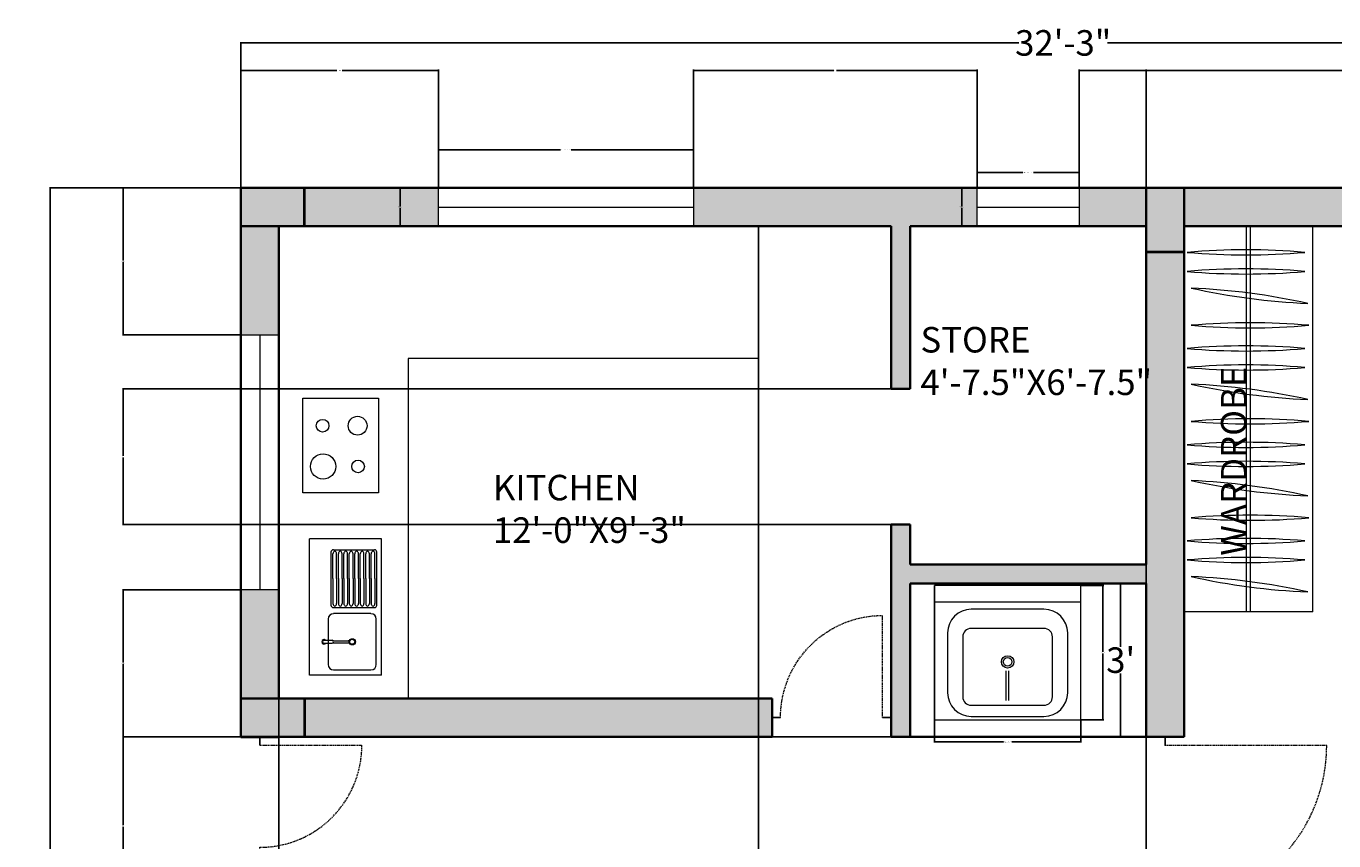
# Model space of a CAD drawing. Units: inches. Extents: x -10 to 455, y -513 to 57.
# Tile 3 of 4: x -10 to 297, y -134 to 57. Entities that reach past the tile are written whole.
import ezdxf

# ---------------------------------------------------------------- set-up
doc = ezdxf.new("R2010")
doc.units = ezdxf.units.IN
doc.header["$MEASUREMENT"] = 0
doc.linetypes.add('DASHED2', pattern=[0.375, 0.25, -0.125])
for name, color, linetype, lineweight in [('A-ANNO-DIMS', 2, 'Continuous', 18), ('A-ANNO-TEXT', 7, 'Continuous', 18), ('A-AREA-IDEN', 7, 'Continuous', 18), ('A-COLS', 7, 'Continuous', 40), ('A-COLS-PATT', 1, 'Continuous', 13), ('A-DOOR', 40, 'DASHED2', 18), ('A-DOOR-FRAM', 7, 'Continuous', 25), ('A-EQPM', 9, 'Continuous', 18), ('A-FLOR-CASE', 8, 'Continuous', 18), ('A-FLOR-FIXT', 9, 'Continuous', 18), ('A-GLAZ', 222, 'Continuous', 18), ('A-WALL', 7, 'Continuous', 35), ('A-WALL-PATT', 152, 'Continuous', 13)]:
    doc.layers.add(name, color=color, linetype=linetype, lineweight=lineweight)
doc.styles.get("Standard").update_dxf_attribs({"font": 'arial.ttf'})
doc.dimstyles.get("Standard").update_dxf_attribs({"dimtxt": 0.18, "dimasz": 0.18, "dimexe": 0.18, "dimexo": 0.0625, "dimgap": 0.09, "dimtad": 0, "dimtih": 1, "dimtoh": 1, "dimdec": 0, "dimzin": 0, "dimdsep": 46, "dimlunit": 3, "dimtxsty": 'Standard', "dimcen": 0.09, "dimadec": 0, "dimazin": 0, "dimtfac": 1, "dimtdec": 0, "dimtofl": 0, "dimtmove": 0, "dimatfit": 3, "dimfxl": 1, "dimtolj": 1, "dimtzin": 0, "dimarcsym": 0})

# ---------------------------------------------------------------- blocks, each defined once
blk = doc.blocks.new('*D1')
at = {"layer": 'A-ANNO-DIMS', "color": 0, "lineweight": -2, "transparency": 16777216}
for p, q in [((40.25, 19.21), (40.25, 53.43)), ((40.43, 53.25), (223.35, 53.25)), ((427.07, 53.25), (244.14, 53.25)), ((427.25, 19.21), (427.25, 53.43))]:
    blk.add_line(p, q, dxfattribs=at)
at = {"layer": 'A-ANNO-DIMS', "color": 0, "transparency": 16777216}
for points in [[(40.43, 53.28), (40.43, 53.22), (40.25, 53.25)], [(427.07, 53.28), (427.07, 53.22), (427.25, 53.25)]]:
    blk.add_solid(points, dxfattribs=at)
at = {"layer": 'Defpoints', "color": 0, "transparency": 16777216}
for p in [(427.25, 53.25), (40.25, 19.15), (427.25, 19.15)]:
    blk.add_point(p, dxfattribs=at)
at = {"layer": 'A-ANNO-DIMS', "color": 0, "transparency": 16777216, "insert": (233.75, 53.25), "char_height": 6, "attachment_point": 5}
blk.add_mtext('\\A1;32\'-3"', dxfattribs=at)
blk = doc.blocks.new('*D2')
at = {"layer": 'A-ANNO-DIMS', "color": 0, "lineweight": -2, "transparency": 16777216}
for p, q in [((40.18, 19.15), (-4.74, 19.15)), ((-4.56, 18.97), (-4.56, -229.75)), ((-4.56, -484.67), (-4.56, -235.95)), ((40.18, -484.85), (-4.74, -484.85))]:
    blk.add_line(p, q, dxfattribs=at)
at = {"layer": 'A-ANNO-DIMS', "color": 0, "transparency": 16777216}
for points in [[(-4.59, 18.97), (-4.53, 18.97), (-4.56, 19.15)], [(-4.59, -484.67), (-4.53, -484.67), (-4.56, -484.85)]]:
    blk.add_solid(points, dxfattribs=at)
at = {"layer": 'Defpoints', "color": 0, "transparency": 16777216}
for p in [(40.25, 19.15), (-4.56, -484.85), (40.25, -484.85)]:
    blk.add_point(p, dxfattribs=at)
at = {"layer": 'A-ANNO-DIMS', "color": 0, "transparency": 16777216, "insert": (-4.56, -232.85), "char_height": 6, "attachment_point": 5}
blk.add_mtext("\\A1;42'", dxfattribs=at)
blk = doc.blocks.new('*D4')
at = {"layer": 'A-ANNO-DIMS', "color": 0, "lineweight": -2, "transparency": 16777216}
for p, q in [((247.27, -74.03), (247.27, -88.69)), ((247.34, -73.85), (247.45, -73.85)), ((247.27, -109.67), (247.27, -95.01)), ((247.34, -109.85), (247.45, -109.85))]:
    blk.add_line(p, q, dxfattribs=at)
at = {"layer": 'A-ANNO-DIMS', "color": 0, "transparency": 16777216}
for points in [[(247.24, -74.03), (247.3, -74.03), (247.27, -73.85)], [(247.24, -109.67), (247.3, -109.67), (247.27, -109.85)]]:
    blk.add_solid(points, dxfattribs=at)
at = {"layer": 'Defpoints', "color": 0, "transparency": 16777216}
for p in [(247.27, -73.85), (247.27, -109.85), (247.27, -109.85)]:
    blk.add_point(p, dxfattribs=at)
at = {"layer": 'A-ANNO-DIMS', "color": 0, "transparency": 16777216, "insert": (247.27, -91.85), "char_height": 6, "attachment_point": 5}
blk.add_mtext("\\A1;3'", dxfattribs=at)
blk = doc.blocks.new('М14 600х655')
for p, q in [((-655, 600), (-655, 0)), ((-655, 600), (-655, 0)), ((-655, 0), (-655, 600)), ((0, 600), (-655, 600)), ((0, 0), (0, 600)), ((0, 525), (-655, 525)), ((-165.1, 494.1), (-489.9, 494.1)), ((-595.8, 388.1), (-595.8, 121.3)), ((-528.4, 370.1), (-528.4, 103.3)), ((-165.4, 408.4), (-490.2, 408.4)), ((-127.2, 103.3), (-127.2, 370.1)), ((-59.2, 121.3), (-59.2, 388.1)), ((-333.5, 87.1), (-333.5, 219.6)), ((-321.5, 87.1), (-321.5, 219.6)), ((-490.2, 65.1), (-165.4, 65.1)), ((-655, 0), (-655, 0)), ((-655, 0), (-655, 0)), ((-655, 0), (0, 0)), ((-655, 0), (0, 0)), ((-489.9, 15.4), (-165.1, 15.4))]:
    blk.add_line(p, q)
for radius in [27.6, 19.3]:
    blk.add_circle((-327.5, 258.9), radius)
for centre, radius, start, end in [((-489.9, 388.1), 105.9, 90, 180), ((-165.1, 388.1), 105.9, 0, 90), ((-490.2, 370.1), 38.2, 90, 180), ((-165.4, 370.1), 38.2, 0, 90), ((-489.9, 121.3), 105.9, 180, 270), ((-165.1, 121.3), 105.9, 270, 0), ((-490.2, 103.3), 38.2, 180, 270), ((-165.4, 103.3), 38.2, 270, 0)]:
    blk.add_arc(centre, radius, start, end)
blk = doc.blocks.new('WIN-60IN')
for p, q in [((0, 9), (60, 9)), ((0, 0), (0, 9)), ((60, 9), (60, 0)), ((0, 4.5), (60, 4.5)), ((60, 0), (0, 0))]:
    blk.add_line(p, q)
blk = doc.blocks.new('WIN-24IN')
for p, q in [((0, 9), (24, 9)), ((0, 0), (0, 9)), ((24, 9), (24, 0)), ((0, 4.5), (24, 4.5)), ((24, 0), (0, 0))]:
    blk.add_line(p, q)
blk = doc.blocks.new('DOOR-SINGLE-24IN')
for p, q in [((0, 28), (0, 26)), ((0, 26), (24, 26)), ((0, 0), (0, 2))]:
    blk.add_line(p, q)
blk.add_arc((0, 26), 24, 270, 0)
blk = doc.blocks.new('*D14')
at = {"layer": 'A-ANNO-DIMS', "color": 0, "lineweight": -2, "transparency": 16777216}
for p, q in [((86.75, 19.21), (86.75, 28.33)), ((86.93, 28.15), (115.52, 28.15)), ((146.57, 28.15), (117.98, 28.15)), ((146.75, 19.21), (146.75, 28.33))]:
    blk.add_line(p, q, dxfattribs=at)
at = {"layer": 'A-ANNO-DIMS', "color": 0, "transparency": 16777216}
for points in [[(86.93, 28.18), (86.93, 28.12), (86.75, 28.15)], [(146.57, 28.18), (146.57, 28.12), (146.75, 28.15)]]:
    blk.add_solid(points, dxfattribs=at)
at = {"layer": 'Defpoints', "color": 0, "transparency": 16777216}
for p in [(146.75, 28.15), (86.75, 19.15), (146.75, 19.15)]:
    blk.add_point(p, dxfattribs=at)
at = {"layer": 'A-ANNO-DIMS', "color": 0, "transparency": 16777216, "insert": (116.75, 28.15), "char_height": 0.18, "attachment_point": 5}
blk.add_mtext('\\A1;WINDOW 5\'-0" TYP.', dxfattribs=at)
blk = doc.blocks.new('*D15')
at = {"layer": 'A-ANNO-DIMS', "color": 0, "lineweight": -2, "transparency": 16777216}
for p, q in [((86.68, 19.15), (77.57, 19.15)), ((77.75, 18.97), (77.75, 14.83)), ((77.75, 10.33), (77.75, 14.47)), ((86.68, 10.15), (77.57, 10.15))]:
    blk.add_line(p, q, dxfattribs=at)
at = {"layer": 'A-ANNO-DIMS', "color": 0, "transparency": 16777216}
for points in [[(77.72, 18.97), (77.78, 18.97), (77.75, 19.15)], [(77.72, 10.33), (77.78, 10.33), (77.75, 10.15)]]:
    blk.add_solid(points, dxfattribs=at)
at = {"layer": 'Defpoints', "color": 0, "transparency": 16777216}
for p in [(77.75, 19.15), (86.75, 19.15), (86.75, 10.15)]:
    blk.add_point(p, dxfattribs=at)
at = {"layer": 'A-ANNO-DIMS', "color": 0, "transparency": 16777216, "insert": (77.75, 14.65), "char_height": 0.18, "attachment_point": 5}
blk.add_mtext('\\A1;0\'-9" TYP.', dxfattribs=at)
blk = doc.blocks.new('*D18')
at = {"layer": 'A-ANNO-DIMS', "color": 0, "lineweight": -2, "transparency": 16777216}
for p, q in [((203.44, -105.95), (203.44, -111.25)), ((237.93, -105.95), (237.93, -111.25)), ((203.62, -111.07), (219.67, -111.07)), ((237.75, -111.07), (221.7, -111.07))]:
    blk.add_line(p, q, dxfattribs=at)
at = {"layer": 'A-ANNO-DIMS', "color": 0, "transparency": 16777216}
for points in [[(203.62, -111.04), (203.62, -111.1), (203.44, -111.07)], [(237.75, -111.04), (237.75, -111.1), (237.93, -111.07)]]:
    blk.add_solid(points, dxfattribs=at)
at = {"layer": 'Defpoints', "color": 0, "transparency": 16777216}
for p in [(203.44, -105.89), (237.93, -105.89), (237.93, -111.07)]:
    blk.add_point(p, dxfattribs=at)
at = {"layer": 'A-ANNO-DIMS', "color": 0, "transparency": 16777216, "insert": (220.69, -111.07), "char_height": 0.18, "attachment_point": 5}
blk.add_mtext('\\A1;BASIN 2\'-10 1/2"', dxfattribs=at)
blk = doc.blocks.new('*D19')
at = {"layer": 'A-ANNO-DIMS', "color": 0, "lineweight": -2, "transparency": 16777216}
for p, q in [((237.99, -74.3), (243.28, -74.3)), ((243.1, -74.48), (243.1, -89.91)), ((243.1, -105.71), (243.1, -90.28)), ((237.99, -105.89), (243.28, -105.89))]:
    blk.add_line(p, q, dxfattribs=at)
at = {"layer": 'A-ANNO-DIMS', "color": 0, "transparency": 16777216}
for points in [[(243.07, -74.48), (243.13, -74.48), (243.1, -74.3)], [(243.07, -105.71), (243.13, -105.71), (243.1, -105.89)]]:
    blk.add_solid(points, dxfattribs=at)
at = {"layer": 'Defpoints', "color": 0, "transparency": 16777216}
for p in [(237.93, -74.3), (243.1, -74.3), (237.93, -105.89)]:
    blk.add_point(p, dxfattribs=at)
at = {"layer": 'A-ANNO-DIMS', "color": 0, "transparency": 16777216, "insert": (243.1, -90.09), "char_height": 0.18, "attachment_point": 5}
blk.add_mtext('\\A1;2\'-7 1/2"', dxfattribs=at)
blk = doc.blocks.new('*D22')
at = {"layer": 'A-ANNO-DIMS', "color": 0, "lineweight": -2, "transparency": 16777216}
for p, q in [((213.5, 19.21), (213.5, 22.93)), ((213.68, 22.75), (224.27, 22.75)), ((237.32, 22.75), (226.73, 22.75)), ((237.5, 19.21), (237.5, 22.93))]:
    blk.add_line(p, q, dxfattribs=at)
at = {"layer": 'A-ANNO-DIMS', "color": 0, "transparency": 16777216}
for points in [[(213.68, 22.78), (213.68, 22.72), (213.5, 22.75)], [(237.32, 22.78), (237.32, 22.72), (237.5, 22.75)]]:
    blk.add_solid(points, dxfattribs=at)
at = {"layer": 'Defpoints', "color": 0, "transparency": 16777216}
for p in [(237.5, 22.75), (213.5, 19.15), (237.5, 19.15)]:
    blk.add_point(p, dxfattribs=at)
at = {"layer": 'A-ANNO-DIMS', "color": 0, "transparency": 16777216, "insert": (225.5, 22.75), "char_height": 0.18, "attachment_point": 5}
blk.add_mtext('\\A1;WINDOW 2\'-0" TYP.', dxfattribs=at)
blk = doc.blocks.new('*D23')
at = {"layer": 'A-ANNO-DIMS', "color": 0, "lineweight": -2, "transparency": 16777216}
for p, q in [((213.43, 19.15), (209.72, 19.15)), ((209.9, 18.97), (209.9, 14.83)), ((209.9, 10.33), (209.9, 14.47)), ((213.43, 10.15), (209.72, 10.15))]:
    blk.add_line(p, q, dxfattribs=at)
at = {"layer": 'A-ANNO-DIMS', "color": 0, "transparency": 16777216}
for points in [[(209.87, 18.97), (209.93, 18.97), (209.9, 19.15)], [(209.87, 10.33), (209.93, 10.33), (209.9, 10.15)]]:
    blk.add_solid(points, dxfattribs=at)
at = {"layer": 'Defpoints', "color": 0, "transparency": 16777216}
for p in [(209.9, 19.15), (213.5, 19.15), (213.5, 10.15)]:
    blk.add_point(p, dxfattribs=at)
at = {"layer": 'A-ANNO-DIMS', "color": 0, "transparency": 16777216, "insert": (209.9, 14.65), "char_height": 0.18, "attachment_point": 5}
blk.add_mtext('\\A1;0\'-9" TYP.', dxfattribs=at)
blk = doc.blocks.new('*D30')
at = {"layer": 'A-ANNO-DIMS', "color": 0, "lineweight": -2, "transparency": 16777216}
for p, q in [((40.25, 19.21), (40.25, 46.98)), ((40.43, 46.8), (62.89, 46.8)), ((86.57, 46.8), (64.1, 46.8)), ((86.75, 19.21), (86.75, 46.98))]:
    blk.add_line(p, q, dxfattribs=at)
at = {"layer": 'A-ANNO-DIMS', "color": 0, "transparency": 16777216}
for points in [[(40.43, 46.83), (40.43, 46.77), (40.25, 46.8)], [(86.57, 46.83), (86.57, 46.77), (86.75, 46.8)]]:
    blk.add_solid(points, dxfattribs=at)
at = {"layer": 'Defpoints', "color": 0, "transparency": 16777216}
for p in [(86.75, 46.8), (40.25, 19.15), (86.75, 19.15)]:
    blk.add_point(p, dxfattribs=at)
at = {"layer": 'A-ANNO-DIMS', "color": 0, "transparency": 16777216, "insert": (63.5, 46.8), "char_height": 0.18, "attachment_point": 5}
blk.add_mtext('\\A1;3\'-10 1/2"', dxfattribs=at)
blk = doc.blocks.new('*D31')
at = {"layer": 'A-ANNO-DIMS', "color": 0, "lineweight": -2, "transparency": 16777216}
for p, q in [((146.75, 19.21), (146.75, 46.98)), ((146.93, 46.8), (179.79, 46.8)), ((213.32, 46.8), (180.45, 46.8)), ((213.5, 19.21), (213.5, 46.98))]:
    blk.add_line(p, q, dxfattribs=at)
at = {"layer": 'A-ANNO-DIMS', "color": 0, "transparency": 16777216}
for points in [[(146.93, 46.83), (146.93, 46.77), (146.75, 46.8)], [(213.32, 46.83), (213.32, 46.77), (213.5, 46.8)]]:
    blk.add_solid(points, dxfattribs=at)
at = {"layer": 'Defpoints', "color": 0, "transparency": 16777216}
for p in [(213.5, 46.8), (146.75, 19.15), (213.5, 19.15)]:
    blk.add_point(p, dxfattribs=at)
at = {"layer": 'A-ANNO-DIMS', "color": 0, "transparency": 16777216, "insert": (180.12, 46.8), "char_height": 0.18, "attachment_point": 5}
blk.add_mtext('\\A1;5\'-7"', dxfattribs=at)
blk = doc.blocks.new('*D32')
at = {"layer": 'A-ANNO-DIMS', "color": 0, "lineweight": -2, "transparency": 16777216}
for p, q in [((237.5, 19.21), (237.5, 46.98)), ((237.68, 46.8), (273.54, 46.8)), ((310.07, 46.8), (274.2, 46.8)), ((310.25, 19.21), (310.25, 46.98))]:
    blk.add_line(p, q, dxfattribs=at)
at = {"layer": 'A-ANNO-DIMS', "color": 0, "transparency": 16777216}
for points in [[(237.68, 46.83), (237.68, 46.77), (237.5, 46.8)], [(310.07, 46.83), (310.07, 46.77), (310.25, 46.8)]]:
    blk.add_solid(points, dxfattribs=at)
at = {"layer": 'Defpoints', "color": 0, "transparency": 16777216}
for p in [(310.25, 46.8), (237.5, 19.15), (310.25, 19.15)]:
    blk.add_point(p, dxfattribs=at)
at = {"layer": 'A-ANNO-DIMS', "color": 0, "transparency": 16777216, "insert": (273.87, 46.8), "char_height": 0.18, "attachment_point": 5}
blk.add_mtext('\\A1;6\'-1"', dxfattribs=at)
blk = doc.blocks.new('*D33')
at = {"layer": 'A-ANNO-DIMS', "color": 0, "lineweight": -2, "transparency": 16777216}
for p, q in [((40.18, 19.15), (12.42, 19.15)), ((12.6, 18.97), (12.6, 2.08)), ((12.6, -15.17), (12.6, 1.72)), ((40.18, -15.35), (12.42, -15.35))]:
    blk.add_line(p, q, dxfattribs=at)
at = {"layer": 'A-ANNO-DIMS', "color": 0, "transparency": 16777216}
for points in [[(12.57, 18.97), (12.63, 18.97), (12.6, 19.15)], [(12.57, -15.17), (12.63, -15.17), (12.6, -15.35)]]:
    blk.add_solid(points, dxfattribs=at)
at = {"layer": 'Defpoints', "color": 0, "transparency": 16777216}
for p in [(40.25, 19.15), (12.6, -15.35), (40.25, -15.35)]:
    blk.add_point(p, dxfattribs=at)
at = {"layer": 'A-ANNO-DIMS', "color": 0, "transparency": 16777216, "insert": (12.6, 1.9), "char_height": 0.18, "attachment_point": 5}
blk.add_mtext('\\A1;2\'-10 1/2"', dxfattribs=at)
blk = doc.blocks.new('*D34')
at = {"layer": 'A-ANNO-DIMS', "color": 0, "lineweight": -2, "transparency": 16777216}
for p, q in [((40.18, -75.35), (12.42, -75.35)), ((12.6, -75.53), (12.6, -92.42)), ((12.6, -109.67), (12.6, -92.78)), ((40.18, -109.85), (12.42, -109.85))]:
    blk.add_line(p, q, dxfattribs=at)
at = {"layer": 'A-ANNO-DIMS', "color": 0, "transparency": 16777216}
for points in [[(12.57, -75.53), (12.63, -75.53), (12.6, -75.35)], [(12.57, -109.67), (12.63, -109.67), (12.6, -109.85)]]:
    blk.add_solid(points, dxfattribs=at)
at = {"layer": 'Defpoints', "color": 0, "transparency": 16777216}
for p in [(40.25, -75.35), (12.6, -109.85), (40.25, -109.85)]:
    blk.add_point(p, dxfattribs=at)
at = {"layer": 'A-ANNO-DIMS', "color": 0, "transparency": 16777216, "insert": (12.6, -92.6), "char_height": 0.18, "attachment_point": 5}
blk.add_mtext('\\A1;2\'-10 1/2"', dxfattribs=at)
blk = doc.blocks.new('*D41')
at = {"layer": 'A-ANNO-DIMS', "color": 0, "lineweight": -2, "transparency": 16777216}
for p, q in [((253.25, -160.79), (253.25, 46.98)), ((253.43, 46.8), (307.92, 46.8)), ((363.07, 46.8), (308.58, 46.8)), ((363.25, -160.79), (363.25, 46.98))]:
    blk.add_line(p, q, dxfattribs=at)
at = {"layer": 'A-ANNO-DIMS', "color": 0, "transparency": 16777216}
for points in [[(253.43, 46.83), (253.43, 46.77), (253.25, 46.8)], [(363.07, 46.83), (363.07, 46.77), (363.25, 46.8)]]:
    blk.add_solid(points, dxfattribs=at)
at = {"layer": 'Defpoints', "color": 0, "transparency": 16777216}
for p in [(363.25, 46.8), (253.25, -160.85), (363.25, -160.85)]:
    blk.add_point(p, dxfattribs=at)
at = {"layer": 'A-ANNO-DIMS', "color": 0, "transparency": 16777216, "insert": (308.25, 46.8), "char_height": 0.18, "attachment_point": 5}
blk.add_mtext('\\A1;9\'-2"', dxfattribs=at)
blk = doc.blocks.new('*D42')
at = {"layer": 'A-ANNO-DIMS', "color": 0, "lineweight": -2, "transparency": 16777216}
for p, q in [((193.18, -28.04), (12.42, -28.04)), ((12.6, -28.22), (12.6, -43.84)), ((12.6, -59.82), (12.6, -44.2)), ((193.18, -60), (12.42, -60))]:
    blk.add_line(p, q, dxfattribs=at)
at = {"layer": 'A-ANNO-DIMS', "color": 0, "transparency": 16777216}
for points in [[(12.57, -28.22), (12.63, -28.22), (12.6, -28.04)], [(12.57, -59.82), (12.63, -59.82), (12.6, -60)]]:
    blk.add_solid(points, dxfattribs=at)
at = {"layer": 'Defpoints', "color": 0, "transparency": 16777216}
for p in [(193.25, -28.04), (12.6, -60), (193.25, -60)]:
    blk.add_point(p, dxfattribs=at)
at = {"layer": 'A-ANNO-DIMS', "color": 0, "transparency": 16777216, "insert": (12.6, -44.02), "char_height": 0.18, "attachment_point": 5}
blk.add_mtext('\\A1;2\'-8"', dxfattribs=at)
blk = doc.blocks.new('*D43')
at = {"layer": 'A-ANNO-DIMS', "color": 0, "lineweight": -2, "transparency": 16777216}
for p, q in [((253.18, -109.85), (12.42, -109.85)), ((12.6, -110.03), (12.6, -130.67)), ((12.6, -151.67), (12.6, -131.03)), ((253.18, -151.85), (12.42, -151.85))]:
    blk.add_line(p, q, dxfattribs=at)
at = {"layer": 'A-ANNO-DIMS', "color": 0, "transparency": 16777216}
for points in [[(12.57, -110.03), (12.63, -110.03), (12.6, -109.85)], [(12.57, -151.67), (12.63, -151.67), (12.6, -151.85)]]:
    blk.add_solid(points, dxfattribs=at)
at = {"layer": 'Defpoints', "color": 0, "transparency": 16777216}
for p in [(253.25, -109.85), (12.6, -151.85), (253.25, -151.85)]:
    blk.add_point(p, dxfattribs=at)
at = {"layer": 'A-ANNO-DIMS', "color": 0, "transparency": 16777216, "insert": (12.6, -130.85), "char_height": 0.18, "attachment_point": 5}
blk.add_mtext('\\A1;3\'-6"', dxfattribs=at)
blk = doc.blocks.new('*D44')
at = {"layer": 'A-ANNO-DIMS', "color": 0, "lineweight": -2, "transparency": 16777216}
for p, q in [((49.25, 10.09), (49.25, -512.68)), ((162.09, 10.09), (162.09, -512.68)), ((49.43, -512.5), (105.34, -512.5)), ((161.91, -512.5), (106, -512.5))]:
    blk.add_line(p, q, dxfattribs=at)
at = {"layer": 'A-ANNO-DIMS', "color": 0, "transparency": 16777216}
for points in [[(49.43, -512.47), (49.43, -512.53), (49.25, -512.5)], [(161.91, -512.47), (161.91, -512.53), (162.09, -512.5)]]:
    blk.add_solid(points, dxfattribs=at)
at = {"layer": 'Defpoints', "color": 0, "transparency": 16777216}
for p in [(49.25, 10.15), (162.09, 10.15), (162.09, -512.5)]:
    blk.add_point(p, dxfattribs=at)
at = {"layer": 'A-ANNO-DIMS', "color": 0, "transparency": 16777216, "insert": (105.67, -512.5), "char_height": 0.18, "attachment_point": 5}
blk.add_mtext('\\A1;9\'-5"', dxfattribs=at)
blk = doc.blocks.new('*D45')
at = {"layer": 'A-ANNO-DIMS', "color": 0, "lineweight": -2, "transparency": 16777216}
for p, q in [((257.66, -111.85), (257.84, -111.85)), ((257.75, -111.94), (257.75, -111.76)), ((300.74, -154.84), (284.74, -138.85)), ((300.92, -154.84), (300.74, -154.84))]:
    blk.add_line(p, q, dxfattribs=at)
at = {"layer": 'A-ANNO-DIMS', "color": 0, "transparency": 16777216}
blk.add_solid([(284.76, -138.83), (284.72, -138.87), (284.62, -138.72)], dxfattribs=at)
at = {"layer": 'Defpoints', "color": 0, "transparency": 16777216}
for p in [(257.75, -111.85), (284.62, -138.72)]:
    blk.add_point(p, dxfattribs=at)
at = {"layer": 'A-ANNO-DIMS', "color": 0, "transparency": 16777216, "insert": (301.33, -154.84), "char_height": 0.18, "attachment_point": 5}
blk.add_mtext('\\A1;R3\'-2"', dxfattribs=at)

msp = doc.modelspace()

# ---------------------------------------------------------------- hatches: boundary and pattern name
at = {"layer": 'A-COLS-PATT'}
h = msp.add_hatch(color=256, dxfattribs=at)
h.dxf.hatch_style = 1
h.paths.add_polyline_path([(55.25, 19.15), (40.25, 19.15), (40.25, 10.15), (55.25, 10.15)])
h.paths.add_polyline_path([(262.25, 19.15), (253.25, 19.15), (253.25, 4.15), (262.25, 4.15)])
h.paths.add_polyline_path([(427.25, 19.15), (418.25, 19.15), (418.25, 4.15), (427.25, 4.15)])
h.paths.add_polyline_path([(427.25, -247.85), (418.25, -247.85), (418.25, -262.85), (427.25, -262.85)])
h.paths.add_polyline_path([(268.25, -247.85), (253.25, -247.85), (253.25, -256.85), (268.25, -256.85)])
h.paths.add_polyline_path([(55.25, -247.85), (40.25, -247.85), (40.25, -256.85), (55.25, -256.85)])
h.paths.add_polyline_path([(55.25, -475.85), (49.25, -475.85), (40.25, -475.85), (40.25, -484.85), (55.25, -484.85)])
h.paths.add_polyline_path([(268.25, -475.85), (253.25, -475.85), (253.25, -484.85), (268.25, -484.85)])
h.paths.add_polyline_path([(427.25, -469.85), (418.25, -469.85), (418.25, -484.85), (427.25, -484.85)])
h.paths.add_polyline_path([(55.25, -100.85), (40.25, -100.85), (40.25, -109.85), (55.25, -109.85)])
at = {"layer": 'A-WALL-PATT'}
h = msp.add_hatch(color=256, dxfattribs=at)
h.dxf.hatch_style = 1
h.paths.add_polyline_path([(418.25, -151.85), (268.25, -151.85), (268.25, -160.85), (418.25, -160.85)])
h.paths.add_polyline_path([(165.25, -100.85), (55.25, -100.85), (55.25, -109.85), (165.25, -109.85), (165.25, -105.35)])
h.paths.add_polyline_path([(49.25, -75.35), (40.25, -75.35), (40.25, -100.85), (49.25, -100.85)])
h.paths.add_polyline_path([(49.25, 10.15), (40.25, 10.15), (40.25, -15.35), (49.25, -15.35)])
h.paths.add_polyline_path([(86.75, 19.15), (55.25, 19.15), (55.25, 10.15), (86.75, 10.15)])
h.paths.add_polyline_path([(213.5, 19.15), (146.75, 19.15), (146.75, 10.15), (193.25, 10.15), (193.25, -28.04), (197.75, -28.04), (197.75, 10.15), (213.5, 10.15)])
h.paths.add_polyline_path([(262.25, 4.15), (253.25, 4.15), (253.25, -69.35), (197.75, -69.35), (197.75, -60), (193.25, -60), (193.25, -109.85), (197.75, -109.85), (197.75, -73.85), (253.25, -73.85), (253.25, -109.85), (262.25, -109.85)])
h.paths.add_polyline_path([(310.25, 19.15), (262.25, 19.15), (262.25, 10.15), (310.25, 10.15)])
h.paths.add_polyline_path([(253.25, 19.15), (237.5, 19.15), (237.5, 10.15), (253.25, 10.15)])
h.paths.add_polyline_path([(418.25, 19.15), (370.25, 19.15), (370.25, 10.15), (418.25, 10.15)])
h.paths.add_polyline_path([(427.25, 4.15), (418.25, 4.15), (418.25, -42.17), (427.25, -42.17)])
h.paths.add_polyline_path([(427.25, -102.17), (418.25, -102.17), (418.25, -145.85), (427.25, -145.85)])
h.paths.add_polyline_path([(427.25, -160.85), (418.25, -160.85), (418.25, -247.85), (427.25, -247.85)])
h.paths.add_polyline_path([(418.25, -247.85), (365.75, -247.85), (365.75, -256.85), (418.25, -256.85)], flags=17)
h.paths.add_polyline_path([(297.25, -247.85), (268.25, -247.85), (268.25, -256.85), (297.25, -256.85), (297.25, -252.35)], flags=17)
h.paths.add_polyline_path([(427.25, -299.44), (418.25, -299.44), (418.25, -319.85), (370.25, -319.85), (370.25, -284.85), (368, -284.85), (365.75, -284.85), (365.75, -319.85), (329.75, -319.85), (329.75, -247.85), (325.25, -247.85), (325.25, -319.85), (257.75, -319.85), (257.75, -256.85), (253.25, -256.85), (253.25, -324.35), (262.25, -324.35), (418.25, -324.35), (418.25, -363.39), (427.25, -363.39)])
h.paths.add_polyline_path([(262.25, -352.35), (257.75, -352.35), (253.25, -352.35), (253.25, -447.85), (257.75, -447.85), (262.25, -447.85)])
h.paths.add_polyline_path([(305.75, -475.85), (268.25, -475.85), (268.25, -484.85), (305.75, -484.85)])
h.paths.add_polyline_path([(418.25, -475.85), (365.75, -475.85), (365.75, -484.85), (418.25, -484.85)])
h.paths.add_polyline_path([(427.25, -423.39), (418.25, -423.39), (418.25, -469.85), (427.25, -469.85)])
h.paths.add_polyline_path([(202.25, -247.85), (193.25, -247.85), (193.25, -403.85), (49.25, -403.85), (49.25, -360.35), (40.25, -360.35), (40.25, -412.85), (202.25, -412.85)])
h.paths.add_polyline_path([(165.25, -247.85), (55.25, -247.85), (55.25, -256.85), (165.25, -256.85), (165.25, -252.35)], flags=17)
h.paths.add_polyline_path([(49.25, -225.11), (40.25, -225.11), (40.25, -247.85), (49.25, -247.85)])
h.paths.add_polyline_path([(49.25, -256.85), (40.25, -256.85), (40.25, -300.35), (49.25, -300.35)], flags=17)
h.paths.add_polyline_path([(49.25, -137.85), (44.75, -137.85), (40.25, -137.85), (40.25, -165.11), (49.25, -165.11)])

# ---------------------------------------------------------------- linework, layer by layer
at = {"layer": 'A-COLS'}
for p, q in [((55.25, 10.15), (55.25, 19.15)), ((253.25, 4.15), (262.25, 4.15)), ((55.25, -100.85), (55.25, -109.85)), ((40.25, -109.85), (49.25, -109.85))]:
    msp.add_line(p, q, dxfattribs=at)
at = {"layer": 'A-DOOR'}
for p, q in [((257.75, -109.85), (257.75, -111.85)), ((257.75, -111.85), (295.75, -111.85))]:
    msp.add_line(p, q, dxfattribs=at)
msp.add_arc((257.75, -111.85), 38, 270, 0, dxfattribs=at)
at = {"layer": 'A-DOOR-FRAM'}
for p, q in [((167.25, -105.35), (165.25, -105.35)), ((193.25, -105.35), (191.25, -105.35)), ((44.75, -109.85), (44.75, -111.85)), ((257.75, -109.85), (257.75, -111.85))]:
    msp.add_line(p, q, dxfattribs=at)
at = {"layer": 'A-EQPM'}
msp.add_lwpolyline([(72.65, -30.26), (72.65, -52.51), (54.85, -52.51), (54.85, -30.26)], close=True, dxfattribs=at)
for centre, radius in [((59.5, -36.74), 1.48), ((67.74, -36.74), 2.22), ((59.63, -46.32), 2.97), ((67.86, -46.32), 1.48)]:
    msp.add_circle(centre, radius, dxfattribs=at)
at = {"layer": 'A-FLOR-CASE'}
for p, q in [((162.09, 10.15), (162.09, -20.94)), ((262.25, -80.48), (262.25, 10.15)), ((292.46, 10.15), (262.25, 10.15)), ((276.85, -80.48), (276.85, 10.15)), ((277.85, -80.48), (277.85, 10.15)), ((292.46, -80.48), (292.46, 10.15)), ((162.09, -20.94), (79.62, -20.94)), ((79.62, -20.94), (79.62, -100.85)), ((292.46, -80.48), (262.25, -80.48))]:
    msp.add_line(p, q, dxfattribs=at)
for centre, start, end in [((276.75, -154.34), 85.0028, 94.9972), ((276.75, 162.35), 265.0028, 274.9972), ((276.75, -158.82), 85.0028, 94.9972), ((276.75, 157.87), 265.0028, 274.9972), ((298.25, 150.8), 257.508, 267.5023), ((256.94, -163.19), 77.508, 87.5023), ((277.72, -171.48), 85.0028, 94.9972), ((277.72, 145.21), 265.0028, 274.9972), ((276.75, -176.92), 85.0028, 94.9972), ((276.75, 139.77), 265.0028, 274.9972), ((276.75, -181.4), 85.0028, 94.9972), ((276.75, 135.3), 265.0028, 274.9972), ((298.25, 128.22), 257.508, 267.5023), ((256.94, -185.77), 77.508, 87.5023), ((277.72, -194.06), 85.0028, 94.9972), ((277.72, 122.63), 265.0028, 274.9972), ((276.75, -199.59), 85.0028, 94.9972), ((276.75, 117.11), 265.0028, 274.9972), ((276.75, -204.06), 85.0028, 94.9972), ((276.75, 112.63), 265.0028, 274.9972), ((256.94, -208.43), 77.508, 87.5023), ((298.25, 105.56), 257.508, 267.5023), ((277.72, -216.73), 85.0028, 94.9972), ((277.72, 99.97), 265.0028, 274.9972), ((276.75, -222.17), 85.0028, 94.9972), ((276.75, 94.53), 265.0028, 274.9972), ((276.75, -226.64), 85.0028, 94.9972), ((276.75, 90.05), 265.0028, 274.9972), ((256.94, -231.01), 77.508, 87.5023), ((298.25, 82.98), 257.508, 267.5023)]:
    msp.add_arc(centre, 158.95, start, end, dxfattribs=at)
at = {"layer": 'A-FLOR-FIXT'}
for p, q in [((73.33, -63.35), (56.4, -63.35)), ((56.4, -95.38), (56.4, -63.35)), ((73.33, -95.38), (73.33, -63.35)), ((61.47, -66.48), (61.47, -78.91)), ((61.94, -72.69), (61.94, -66.83)), ((62.06, -65.89), (71.69, -65.89)), ((62.81, -72.69), (62.81, -66.83)), ((63.22, -72.69), (63.22, -66.83)), ((64.1, -72.69), (64.1, -66.83)), ((64.51, -72.69), (64.51, -66.83)), ((65.38, -72.69), (65.38, -66.83)), ((65.79, -72.69), (65.79, -66.83)), ((66.67, -72.69), (66.67, -66.83)), ((67.08, -72.69), (67.08, -66.83)), ((67.96, -72.69), (67.96, -66.83)), ((68.37, -72.69), (68.37, -66.83)), ((69.24, -72.69), (69.24, -66.83)), ((69.65, -72.69), (69.65, -66.83)), ((70.53, -72.69), (70.53, -66.83)), ((70.94, -72.69), (70.94, -66.83)), ((71.81, -72.69), (71.81, -66.83)), ((72.28, -78.91), (72.28, -66.48)), ((61.94, -72.69), (61.94, -78.56)), ((62.81, -72.69), (62.81, -78.56)), ((63.22, -72.69), (63.22, -78.56)), ((64.1, -72.69), (64.1, -78.56)), ((64.51, -72.69), (64.51, -78.56)), ((65.38, -72.69), (65.38, -78.56)), ((65.79, -72.69), (65.79, -78.56)), ((66.67, -72.69), (66.67, -78.56)), ((67.08, -72.69), (67.08, -78.56)), ((67.96, -72.69), (67.96, -78.56)), ((68.37, -72.69), (68.37, -78.56)), ((69.24, -72.69), (69.24, -78.56)), ((69.65, -72.69), (69.65, -78.56)), ((70.53, -72.69), (70.53, -78.56)), ((70.94, -72.69), (70.94, -78.56)), ((71.81, -72.69), (71.81, -78.56)), ((62.06, -79.49), (71.69, -79.49)), ((60.83, -82.19), (60.83, -87.19)), ((70.89, -80.92), (62.09, -80.92)), ((72.15, -92.89), (72.15, -82.19)), ((60.83, -87.34), (60.83, -92.89)), ((62.09, -94.15), (70.89, -94.15)), ((73.33, -95.38), (56.4, -95.38))]:
    msp.add_line(p, q, dxfattribs=at)
for points in [[(59.84, -87.19), (61.77, -87.19)], [(59.84, -87.89), (61.77, -87.89)], [(61.99, -87.28), (65.53, -87.28)], [(61.99, -87.8), (65.53, -87.8)]]:
    msp.add_lwpolyline(points, dxfattribs=at)
for radius in [0.73, 0.584]:
    msp.add_circle((66.49, -87.54), radius, dxfattribs=at)
for centre, radius, start, end in [((62.06, -66.48), 0.584, 90, 180), ((62.52, -66.83), 0.584, 104.4903, 180), ((62.23, -66.83), 0.584, 0, 75.5097), ((63.81, -66.83), 0.584, 104.4903, 180), ((63.52, -66.83), 0.584, 0, 75.5097), ((65.09, -66.83), 0.584, 104.4903, 180), ((64.8, -66.83), 0.584, 0, 75.5097), ((66.38, -66.83), 0.584, 104.4903, 180), ((66.09, -66.83), 0.584, 0, 75.5097), ((67.66, -66.83), 0.584, 104.4903, 180), ((67.37, -66.83), 0.584, 0, 75.5097), ((68.95, -66.83), 0.584, 104.4903, 180), ((68.66, -66.83), 0.584, 0, 75.5097), ((70.23, -66.83), 0.584, 104.4903, 180), ((69.94, -66.83), 0.584, 0, 75.5097), ((71.52, -66.83), 0.584, 104.4903, 180), ((71.23, -66.83), 0.584, 0, 75.5097), ((71.69, -66.48), 0.584, 0, 90), ((62.06, -78.91), 0.584, 180, 270), ((62.52, -78.56), 0.584, 180, 255.5097), ((62.23, -78.56), 0.584, 284.4903, 0), ((63.81, -78.56), 0.584, 180, 255.5097), ((63.52, -78.56), 0.584, 284.4903, 0), ((65.09, -78.56), 0.584, 180, 255.5097), ((64.8, -78.56), 0.584, 284.4903, 0), ((66.38, -78.56), 0.584, 180, 255.5097), ((66.09, -78.56), 0.584, 284.4903, 0), ((67.66, -78.56), 0.584, 180, 255.5097), ((67.37, -78.56), 0.584, 284.4903, 0), ((68.95, -78.56), 0.584, 180, 255.5097), ((68.66, -78.56), 0.584, 284.4903, 0), ((70.23, -78.56), 0.584, 180, 255.5097), ((69.94, -78.56), 0.584, 284.4903, 0), ((71.52, -78.56), 0.584, 180, 255.5097), ((71.23, -78.56), 0.584, 284.4903, 0), ((71.69, -78.91), 0.584, 270, 0), ((62.09, -82.19), 1.26, 90, 180), ((70.89, -82.19), 1.26, 0, 90), ((59.84, -87.54), 0.524, 41.9018, 318.0982), ((59.84, -87.54), 0.35, 90, 270), ((61.76, -87.54), 0.351, 272.2198, 87.7802), ((65.55, -87.54), 0.264, 264.9463, 95.0537), ((62.09, -92.89), 1.26, 180, 270), ((70.89, -92.89), 1.26, 270, 0)]:
    msp.add_arc(centre, radius, start, end, dxfattribs=at)
at = {"layer": 'A-WALL'}
for p, q in [((40.25, 19.15), (40.25, -109.85)), ((40.25, 19.15), (427.25, 19.15)), ((253.25, 19.15), (253.25, -69.35)), ((262.25, 19.15), (262.25, -109.85)), ((40.25, 10.15), (193.25, 10.15)), ((49.25, 10.15), (49.25, -100.85)), ((193.25, 10.15), (193.25, -28.04)), ((197.75, 10.15), (197.75, -28.04)), ((197.75, 10.15), (253.25, 10.15)), ((262.25, 10.15), (418.25, 10.15)), ((193.25, -28.04), (197.75, -28.04)), ((197.75, -60), (193.25, -60)), ((193.25, -60), (193.25, -109.85)), ((197.75, -60), (197.75, -69.35)), ((197.75, -69.35), (253.25, -69.35)), ((197.75, -73.85), (253.25, -73.85)), ((197.75, -73.85), (197.75, -109.85)), ((253.25, -73.85), (253.25, -109.85)), ((40.25, -100.85), (165.25, -100.85)), ((165.25, -105.35), (165.25, -100.85)), ((193.25, -100.85), (193.25, -109.85)), ((165.25, -105.35), (165.25, -109.85)), ((40.25, -109.85), (165.25, -109.85)), ((193.25, -109.85), (262.25, -109.85)), ((253.25, -109.85), (262.25, -109.85))]:
    msp.add_line(p, q, dxfattribs=at)

# ---------------------------------------------------------------- block references
at = {"layer": 'A-DOOR', "extrusion": (0, 0, -1), "zscale": -1, "rotation": 90.00000000000003}
msp.add_blockref('DOOR-SINGLE-24IN', (-165.25, -105.35), dxfattribs=at)
at = {"layer": 'A-DOOR'}
msp.add_blockref('DOOR-SINGLE-24IN', (44.75, -137.85), dxfattribs=at)
at = {"layer": 'A-FLOR-FIXT', "xscale": 0.0526586176379125, "yscale": 0.0526586176379125, "zscale": 0.0526586176379125}
msp.add_blockref('М14 600х655', (237.93, -105.89), dxfattribs=at)
at = {"layer": 'A-GLAZ'}
for name, p in [('WIN-60IN', (86.75, 10.15)), ('WIN-24IN', (213.5, 10.15))]:
    msp.add_blockref(name, p, dxfattribs=at)
at = {"layer": 'A-GLAZ', "rotation": 270}
msp.add_blockref('WIN-60IN', (40.25, -15.35), dxfattribs=at)

# ---------------------------------------------------------------- texts
at = {"layer": 'A-ANNO-TEXT', "insert": (270.89, -67.31), "char_height": 6, "attachment_point": 1, "rotation": 90}
msp.add_mtext('WARDROBE', dxfattribs=at)
at = {"layer": 'A-AREA-IDEN', "char_height": 6, "attachment_point": 1}
for s, insert in [('STORE\\P4\'-7.5"X6\'-7.5"', (200.17, -13.53)), ('KITCHEN\\P12\'-0"X9\'-3"', (99.58, -48.29))]:
    msp.add_mtext(s, dxfattribs=dict(at, insert=insert))

# ---------------------------------------------------------------- dimensions: what is measured, and where the dimension line sits
at = {"layer": 'A-ANNO-DIMS'}
for base, p1, p2, override, picture, middle in [((427.25, 53.25), (40.25, 19.15), (427.25, 19.15), {"dimtxt": 6, "dimclrd": 0, "dimclre": 0, "dimclrt": 0}, '*D1', (233.75, 53.25)), ((86.75, 46.8), (40.25, 19.15), (86.75, 19.15), {"dimdec": 1, "dimlfac": 1, "dimrnd": 0, "dimzin": 1, "dimdsep": 46, "dimlunit": 4, "dimfrac": 2}, '*D30', (63.5, 46.8)), ((213.496151, 46.799546), (146.746151, 19.149546), (213.496151, 19.149546), {"dimdec": 1, "dimlfac": 1, "dimrnd": 0, "dimzin": 1, "dimdsep": 46, "dimlunit": 4, "dimfrac": 2}, '*D31', (180.121151, 46.799546)), ((310.246151, 46.799546), (237.496151, 19.149546), (310.246151, 19.149546), {"dimdec": 1, "dimlfac": 1, "dimrnd": 0, "dimzin": 1, "dimdsep": 46, "dimlunit": 4, "dimfrac": 2}, '*D32', (273.871151, 46.799546)), ((363.25, 46.8), (253.25, -160.85), (363.25, -160.85), {"dimdec": 1, "dimlfac": 1, "dimrnd": 0, "dimzin": 1, "dimdsep": 46, "dimlunit": 4, "dimfrac": 2}, '*D41', (308.25, 46.8)), ((162.09, -512.5), (49.25, 10.15), (162.09, 10.15), {"dimdec": 1, "dimlfac": 1, "dimrnd": 0, "dimzin": 1, "dimdsep": 46, "dimlunit": 4, "dimfrac": 2}, '*D44', (105.67, -512.5))]:
    dim = msp.add_linear_dim(base=base, p1=p1, p2=p2, dimstyle='Standard', override=override, dxfattribs=at)
    dim.commit()
    dim.dimension.update_dxf_attribs({"geometry": picture, "text_midpoint": middle})
for base, p1, p2, text, picture, middle in [((146.75, 28.15), (86.75, 19.15), (146.75, 19.15), 'WINDOW <> TYP.', '*D14', (116.75, 28.15)), ((237.5, 22.75), (213.5, 19.15), (237.5, 19.15), 'WINDOW <> TYP.', '*D22', (225.5, 22.75)), ((237.93, -111.07), (203.44, -105.89), (237.93, -105.89), 'BASIN <>', '*D18', (220.69, -111.07))]:
    dim = msp.add_linear_dim(base=base, p1=p1, p2=p2, text=text, dimstyle='Standard', override={"dimdec": 1, "dimlfac": 1, "dimrnd": 0, "dimzin": 1, "dimdsep": 46, "dimlunit": 4, "dimfrac": 2}, dxfattribs=at)
    dim.commit()
    dim.dimension.update_dxf_attribs({"geometry": picture, "text_midpoint": middle})
for base, p1, p2, override, picture, middle in [((-4.56, -484.85), (40.25, 19.15), (40.25, -484.85), {"dimtxt": 6, "dimclrd": 0, "dimclre": 0, "dimclrt": 0}, '*D2', (-4.56, -232.85)), ((12.6, -15.35), (40.25, 19.15), (40.25, -15.35), {"dimdec": 1, "dimlfac": 1, "dimrnd": 0, "dimzin": 1, "dimdsep": 46, "dimlunit": 4, "dimfrac": 2}, '*D33', (12.6, 1.9)), ((12.6, -60), (193.25, -28.04), (193.25, -60), {"dimdec": 1, "dimlfac": 1, "dimrnd": 0, "dimzin": 1, "dimdsep": 46, "dimlunit": 4, "dimfrac": 2}, '*D42', (12.6, -44.02)), ((12.6, -109.85), (40.25, -75.35), (40.25, -109.85), {"dimdec": 1, "dimlfac": 1, "dimrnd": 0, "dimzin": 1, "dimdsep": 46, "dimlunit": 4, "dimfrac": 2}, '*D34', (12.6, -92.6)), ((243.1, -74.3), (237.93, -105.89), (237.93, -74.3), {"dimdec": 1, "dimlfac": 1, "dimrnd": 0, "dimzin": 1, "dimdsep": 46, "dimlunit": 4, "dimfrac": 2}, '*D19', (243.1, -90.09)), ((247.27, -109.85), (247.27, -73.85), (247.27, -109.85), {"dimtxt": 6, "dimclrd": 0, "dimclre": 0, "dimclrt": 0}, '*D4', (247.27, -91.85)), ((12.6, -151.85), (253.25, -109.85), (253.25, -151.85), {"dimdec": 1, "dimlfac": 1, "dimrnd": 0, "dimzin": 1, "dimdsep": 46, "dimlunit": 4, "dimfrac": 2}, '*D43', (12.6, -130.85))]:
    dim = msp.add_linear_dim(base=base, p1=p1, p2=p2, angle=90, dimstyle='Standard', override=override, dxfattribs=at)
    dim.commit()
    dim.dimension.update_dxf_attribs({"geometry": picture, "text_midpoint": middle})
for base, p1, p2, picture, middle in [((77.75, 19.15), (86.75, 10.15), (86.75, 19.15), '*D15', (77.75, 14.65)), ((209.9, 19.15), (213.5, 10.15), (213.5, 19.15), '*D23', (209.9, 14.65))]:
    dim = msp.add_linear_dim(base=base, p1=p1, p2=p2, angle=90, text='<> TYP.', dimstyle='Standard', override={"dimdec": 1, "dimlfac": 1, "dimrnd": 0, "dimzin": 1, "dimdsep": 46, "dimlunit": 4, "dimfrac": 2}, dxfattribs=at)
    dim.commit()
    dim.dimension.update_dxf_attribs({"geometry": picture, "text_midpoint": middle})
dim = msp.add_radius_dim(center=(257.75, -111.85), mpoint=(284.62, -138.72), dimstyle='Standard', override={"dimdec": 1, "dimlfac": 1, "dimrnd": 0, "dimzin": 1, "dimdsep": 46, "dimlunit": 4, "dimfrac": 2}, dxfattribs=at)
dim.commit()
dim.dimension.update_dxf_attribs({"geometry": '*D45', "text_midpoint": (301.33, -154.84), "dimtype": 164})

doc.saveas('drawing.dxf')
